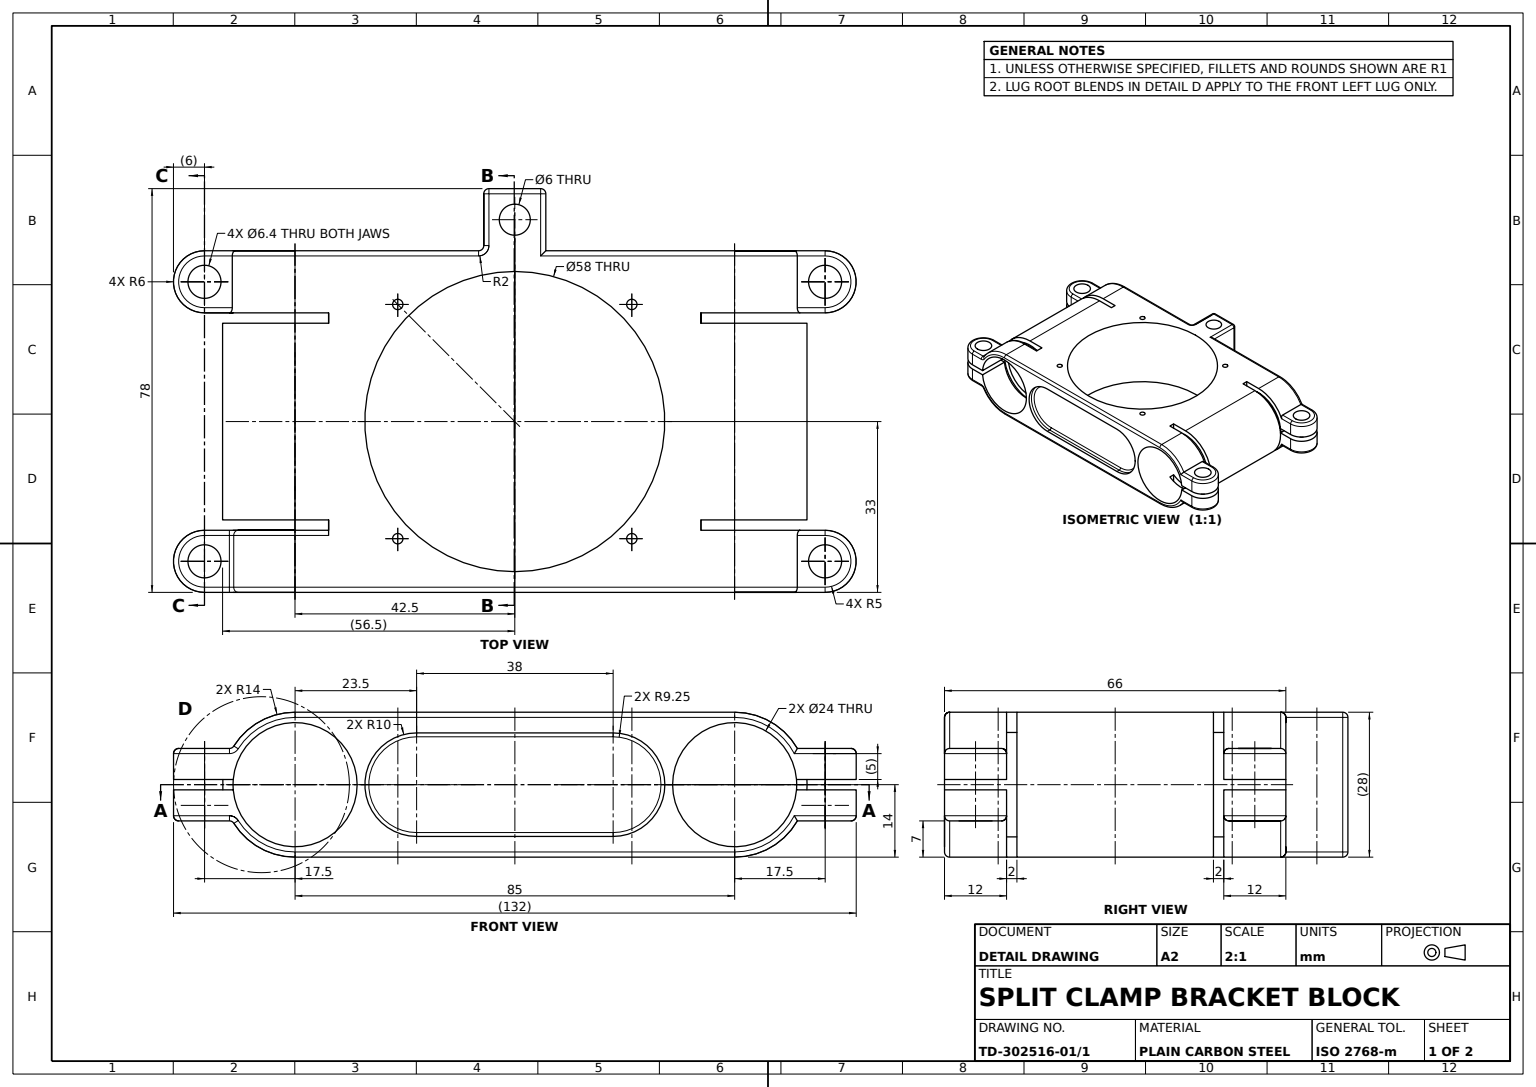
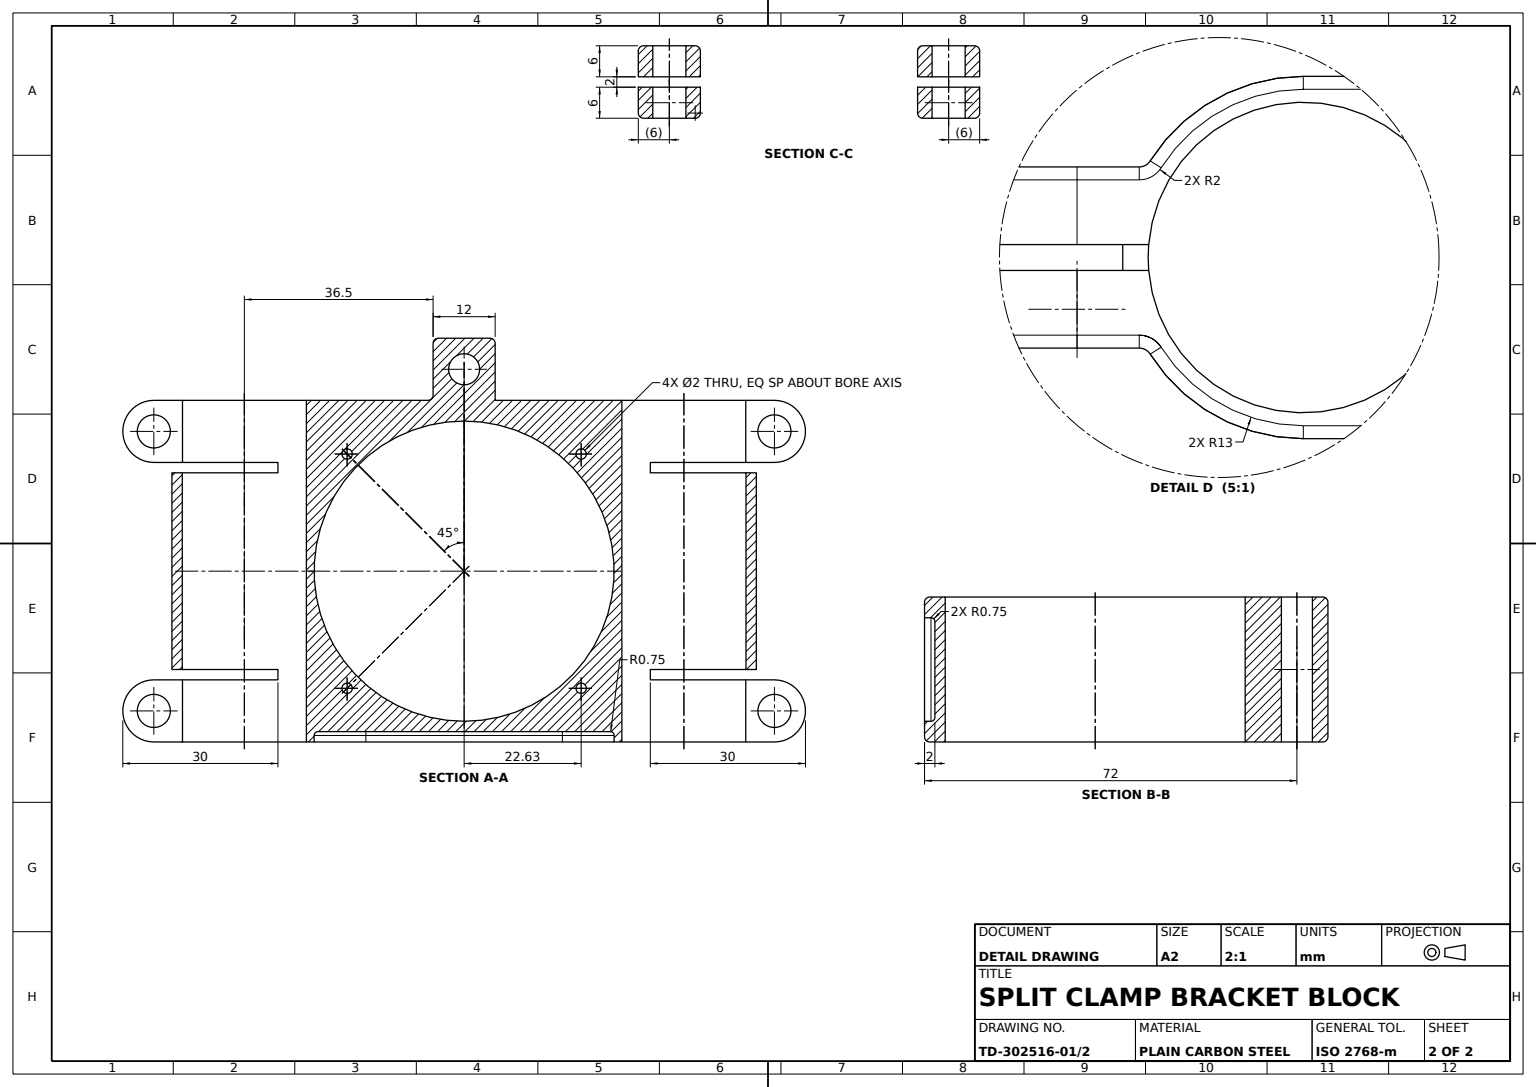
from build123d import *

# Parameters (mm, degrees)
CARRIAGE_BODY_DEPTH                    = 66
ROD_BORE_A_SKETCH_R                    = 12
ROD_BORE_A_24_DEPTH                    = 66
SIDE_POCKET_2MM_DEPTH                  = 2
CENTRE_BORE_SKETCH_R                   = 29
CENTRE_BORE_58_DEPTH                   = 123.233383329
BORE_SCREW_HOLES_SKETCH_R              = 1
BORE_SCREW_HOLES_4X_2_DEPTH            = 123.233383329
CLAMP_LUG_DEPTH                        = 7
LUG_SPLIT_DEPTH                        = 1
LUG_HOLE_SKETCH_R                      = 3.2
LUG_HOLE_6_4_DEPTH                     = 129.721598809
LUG_PAIR_MIRROR_PLANE2_COPY_1_DEPTH    = 7
LUG_PAIR_MIRROR_PLANE2_COPY_2_DEPTH    = 1
LUG_PAIR_MIRROR_PLANE2_COPY_3_SKETCH_R = 3.2
LUG_PAIR_MIRROR_PLANE2_COPY_3_DEPTH    = 129.721598809
ROD_BORE_B_SKETCH_R                    = 12
ROD_BORE_B_24_DEPTH                    = 128.766388381
CLAMP_SPLIT_SLOTS_SKETCH_W             = 30
CLAMP_SPLIT_SLOTS_SKETCH_H             = 2
CLAMP_SPLIT_SLOTS_DEPTH                = 131.04710685
SIDE_TAB_SKETCH_W                      = 12
SIDE_TAB_SKETCH_H                      = 12
SIDE_TAB_DEPTH                         = 28
SIDE_TAB_HOLE_SKETCH_R                 = 3
SIDE_TAB_HOLE_6_DEPTH                  = 28
LUG_EDGE_FILLETS_R1_R                  = 1
SIDE_POCKET_FILLET_R0_75_R             = 0.75


with BuildPart() as part:
    # Body Profile Sketch → Carriage Body (new body)
    with BuildSketch(Plane.XY):
        with BuildLine():
            Line((0, 14), (85, 14))
            ThreePointArc((85, 14), (99, 0), (85, -14))
            Line((85, -14), (0, -14))
            ThreePointArc((0, -14), (-14, 0), (0, 14))
        make_face()
    extrude(amount=-CARRIAGE_BODY_DEPTH)

    # Rod Bore A Sketch → Rod Bore A Ø24 (cut)
    with BuildSketch(Plane.XY):
        Circle(ROD_BORE_A_SKETCH_R)
        with Locations((85, 0)):
            Circle(ROD_BORE_A_SKETCH_R)
    extrude(amount=-ROD_BORE_A_24_DEPTH, mode=Mode.SUBTRACT)

    # Side Pocket Sketch → Side Pocket 2mm (cut)
    with BuildSketch(Plane.XY):
        with BuildLine():
            Line((23.5, 10), (61.5, 10))
            ThreePointArc((61.5, 10), (71.5, 0), (61.5, -10))
            Line((61.5, -10), (23.5, -10))
            ThreePointArc((23.5, -10), (13.5, 0), (23.5, 10))
        make_face()
    extrude(amount=-SIDE_POCKET_2MM_DEPTH, mode=Mode.SUBTRACT)

    # Centre Bore Sketch → Centre Bore Ø58 (cut, through all)
    with BuildSketch(Plane(origin=(0, 14, 0), x_dir=(1, 0, 0), z_dir=(0, 1, 0))):
        with Locations(Location((42.5, 33, 0), (0, 0, 270))):
            Circle(CENTRE_BORE_SKETCH_R)
    extrude(amount=-CENTRE_BORE_58_DEPTH, mode=Mode.SUBTRACT)

    # Bore Screw Holes Sketch → Bore Screw Holes 4xØ2 (cut, through all)
    with BuildSketch(Plane(origin=(0, 14, 0), x_dir=(1, 0, 0), z_dir=(0, 1, 0))):
        with Locations(Location((65.127416998, 55.627416998, 0), (0, 0, 270))):
            Circle(BORE_SCREW_HOLES_SKETCH_R)
        with Locations(Location((65.127416998, 10.372583002, 0), (0, 0, 270))):
            Circle(BORE_SCREW_HOLES_SKETCH_R)
        with Locations(Location((19.872583002, 10.372583002, 0), (0, 0, 270))):
            Circle(BORE_SCREW_HOLES_SKETCH_R)
        with Locations(Location((19.872583002, 55.627416998, 0), (0, 0, 270))):
            Circle(BORE_SCREW_HOLES_SKETCH_R)
    extrude(amount=-BORE_SCREW_HOLES_4X_2_DEPTH, mode=Mode.SUBTRACT)

    # Clamp Lug Sketch → Clamp Lug (add, symmetric)
    with BuildSketch(Plane(origin=(0, 0, 0), x_dir=(1, 0, 0), z_dir=(0, 1, 0))):
        with BuildLine():
            Line((102.5, 12), (96.5, 12))
            Line((96.5, 12), (96.5, 0))
            Line((96.5, 0), (102.5, 0))
            ThreePointArc((102.5, 0), (108.5, 6), (102.5, 12))
        make_face()
    clamp_lug = extrude(amount=CLAMP_LUG_DEPTH, both=True)

    # Lug Split Sketch → Lug Split (cut, symmetric)
    with BuildSketch(Plane(origin=(0, 0, 0), x_dir=(1, 0, 0), z_dir=(0, 1, 0))):
        with BuildLine():
            Line((97.124355653, 0), (102.5, 0))
            ThreePointArc((102.5, 0), (108.5, 6), (102.5, 12))
            Line((102.5, 12), (97.124355653, 12))
            Line((97.124355653, 12), (92.124355653, 12))
            Line((92.124355653, 12), (92.124355653, 0))
            Line((92.124355653, 0), (97.124355653, 0))
        make_face()
    lug_split = extrude(amount=LUG_SPLIT_DEPTH, both=True, mode=Mode.SUBTRACT)

    # Lug Hole Sketch → Lug Hole Ø6.4 (cut, through all)
    with BuildSketch(Plane(origin=(0, 7, 0), x_dir=(1, 0, 0), z_dir=(0, 1, 0))):
        with Locations(Location((102.5, 6, 0), (0, 0, 270))):
            Circle(LUG_HOLE_SKETCH_R)
    lug_hole_6_4 = extrude(amount=-LUG_HOLE_6_4_DEPTH, mode=Mode.SUBTRACT)

    # Lug Mirror Plane2: Clamp Lug, Lug Split, Lug Hole Ø6.4 across plane
    add(clamp_lug.mirror(Plane.XY.offset(-33)))
    add(lug_split.mirror(Plane.XY.offset(-33)), mode=Mode.SUBTRACT)
    add(lug_hole_6_4.mirror(Plane.XY.offset(-33)), mode=Mode.SUBTRACT)

    # Lug Mirror Plane4: Clamp Lug, Lug Split, Lug Hole Ø6.4 across plane
    add(clamp_lug.mirror(Plane(origin=(42.5, 0, 0), x_dir=(0, 0, 1), z_dir=(1, 0, 0))))
    add(lug_split.mirror(Plane(origin=(42.5, 0, 0), x_dir=(0, 0, 1), z_dir=(1, 0, 0))), mode=Mode.SUBTRACT)
    add(lug_hole_6_4.mirror(Plane(origin=(42.5, 0, 0), x_dir=(0, 0, 1), z_dir=(1, 0, 0))), mode=Mode.SUBTRACT)

    # Lug Pair Mirror Plane2: Clamp Lug, Lug Split, Lug Hole Ø6.4 across plane
    add(clamp_lug.mirror(Plane.XY.offset(-33)))
    add(lug_split.mirror(Plane.XY.offset(-33)), mode=Mode.SUBTRACT)
    add(lug_hole_6_4.mirror(Plane.XY.offset(-33)), mode=Mode.SUBTRACT)

    # Lug Pair Mirror Plane2 copy 1 sketch → Lug Pair Mirror Plane2 copy 1 (add, symmetric)
    with BuildSketch(Plane(origin=(85, 0, -66), x_dir=(-1, 0, 0), z_dir=(0, 1, 0))):
        with BuildLine():
            Line((102.5, 12), (96.5, 12))
            Line((96.5, 12), (96.5, 0))
            Line((96.5, 0), (102.5, 0))
            ThreePointArc((102.5, 0), (108.5, 6), (102.5, 12))
        make_face()
    extrude(amount=LUG_PAIR_MIRROR_PLANE2_COPY_1_DEPTH, both=True)

    # Lug Pair Mirror Plane2 copy 2 sketch → Lug Pair Mirror Plane2 copy 2 (cut, symmetric)
    with BuildSketch(Plane(origin=(85, 0, -66), x_dir=(-1, 0, 0), z_dir=(0, 1, 0))):
        with BuildLine():
            Line((97.124355653, 0), (102.5, 0))
            ThreePointArc((102.5, 0), (108.5, 6), (102.5, 12))
            Line((102.5, 12), (97.124355653, 12))
            Line((97.124355653, 12), (92.124355653, 12))
            Line((92.124355653, 12), (92.124355653, 0))
            Line((92.124355653, 0), (97.124355653, 0))
        make_face()
    extrude(amount=LUG_PAIR_MIRROR_PLANE2_COPY_2_DEPTH, both=True, mode=Mode.SUBTRACT)

    # Lug Pair Mirror Plane2 copy 3 sketch → Lug Pair Mirror Plane2 copy 3 (cut, through all)
    with BuildSketch(Plane(origin=(85, 7, -66), x_dir=(-1, 0, 0), z_dir=(0, 1, 0))):
        with Locations(Location((102.5, 6, 0), (0, 0, 270))):
            Circle(LUG_PAIR_MIRROR_PLANE2_COPY_3_SKETCH_R)
    extrude(amount=-LUG_PAIR_MIRROR_PLANE2_COPY_3_DEPTH, mode=Mode.SUBTRACT)

    # Rod Bore B Sketch → Rod Bore B Ø24 (cut, through all)
    with BuildSketch(Plane(origin=(0, 0, -66), x_dir=(-1, 0, 0), z_dir=(0, 0, -1))):
        with Locations(Location((-85, 0, 0), (0, 0, 175.219808153))):
            Circle(ROD_BORE_B_SKETCH_R)
        with Locations(Location((0, 0, 0), (0, 0, 4.780191847))):
            Circle(ROD_BORE_B_SKETCH_R)
    extrude(amount=-ROD_BORE_B_24_DEPTH, mode=Mode.SUBTRACT)

    # Clamp Split Slots Sketch → Clamp Split Slots (cut, through all)
    with BuildSketch(Plane(origin=(0, 14, 0), x_dir=(1, 0, 0), z_dir=(0, 1, 0))):
        with Locations((93.5, 53)):
            Rectangle(CLAMP_SPLIT_SLOTS_SKETCH_W, CLAMP_SPLIT_SLOTS_SKETCH_H)
        with Locations((93.5, 13)):
            Rectangle(CLAMP_SPLIT_SLOTS_SKETCH_W, CLAMP_SPLIT_SLOTS_SKETCH_H)
        with Locations((-8.5, 13)):
            Rectangle(CLAMP_SPLIT_SLOTS_SKETCH_W, CLAMP_SPLIT_SLOTS_SKETCH_H)
        with Locations((-8.5, 53)):
            Rectangle(CLAMP_SPLIT_SLOTS_SKETCH_W, CLAMP_SPLIT_SLOTS_SKETCH_H)
    extrude(amount=-CLAMP_SPLIT_SLOTS_DEPTH, mode=Mode.SUBTRACT)

    # Side Tab Sketch → Side Tab (add)
    with BuildSketch(Plane(origin=(0, 14, 0), x_dir=(1, 0, 0), z_dir=(0, 1, 0))):
        with Locations((42.5, 72)):
            Rectangle(SIDE_TAB_SKETCH_W, SIDE_TAB_SKETCH_H)
    extrude(amount=-SIDE_TAB_DEPTH)

    # Side Tab Hole Sketch → Side Tab Hole Ø6 (cut)
    with BuildSketch(Plane(origin=(0, 14, 0), x_dir=(1, 0, 0), z_dir=(0, 1, 0))):
        with Locations(Location((42.5, 72, 0), (0, 0, 270))):
            Circle(SIDE_TAB_HOLE_SKETCH_R)
    extrude(amount=-SIDE_TAB_HOLE_6_DEPTH, mode=Mode.SUBTRACT)

    # Lug Edge Fillets R1
    lug_edge_fillets_r1_edges = [part.edges().sort_by_distance(p)[0] for p in [
        (92, 12.124355653, -66),
        (92, -12.124355653, -66),
        (108.5, 7, -60),
        (99.812177826, 7, -66),
        (99.812177826, 7, -54),
        (99.812177826, -7, -66),
        (108.5, -7, -60),
        (99.812177826, -7, -54),
        (66.75, 14, -66),
        (-7, -12.124355653, 0),
        (-12.124355653, -7, -6),
        (-12.124355653, 7, -6),
        (-23.5, 7, -6),
        (-14.812177826, 7, 0),
        (-14.812177826, 7, -12),
        (-14.812177826, -7, 0),
        (-23.5, -7, -6),
        (-14.812177826, -7, -12),
        (-7, -12.124355653, -66),
        (-23.5, -7, -60),
        (-14.812177826, -7, -54),
        (-14.812177826, -7, -66),
        (-14.812177826, 7, -54),
        (-14.812177826, 7, -66),
        (-23.5, 7, -60),
        (-7, 12.124355653, -66),
        (42.5, 14, 0),
        (-7, -12.124355653, -12),
        (-7, 12.124355653, -12),
        (3.25, -14, -12),
        (3.25, 14, -12),
        (92, -12.124355653, 0),
        (42.5, -14, 0),
        (66.75, -14, -66),
        (18.25, 14, -66),
        (36.5, -14, -72),
        (36.5, 0, -66),
        (42.5, -14, -78),
        (36.5, 0, -78),
        (48.5, -14, -72),
        (48.5, 0, -78),
        (36.5, 14, -72),
        (48.5, 14, -72),
        (42.5, 14, -78),
        (-7, 12.124355653, 0),
        (92, 12.124355653, 0),
        (108.5, -7, -6),
        (99.812177826, -7, -12),
        (99.812177826, -7, 0),
        (99.812177826, 7, -12),
        (99.812177826, 7, 0),
        (108.5, 7, -6),
        (18.25, -14, -66),
    ]]
    fillet(lug_edge_fillets_r1_edges, radius=LUG_EDGE_FILLETS_R1_R)

    # Side Pocket Fillet R0.75
    side_pocket_fillet_r0_75_edges = [part.edges().sort_by_distance(p)[0] for p in [
        (13.5, 0, -2),
        (42.5, 10, -2),
        (71.5, 0, -2),
        (42.5, -10, -2),
    ]]
    fillet(side_pocket_fillet_r0_75_edges, radius=SIDE_POCKET_FILLET_R0_75_R)


solid = part.part
